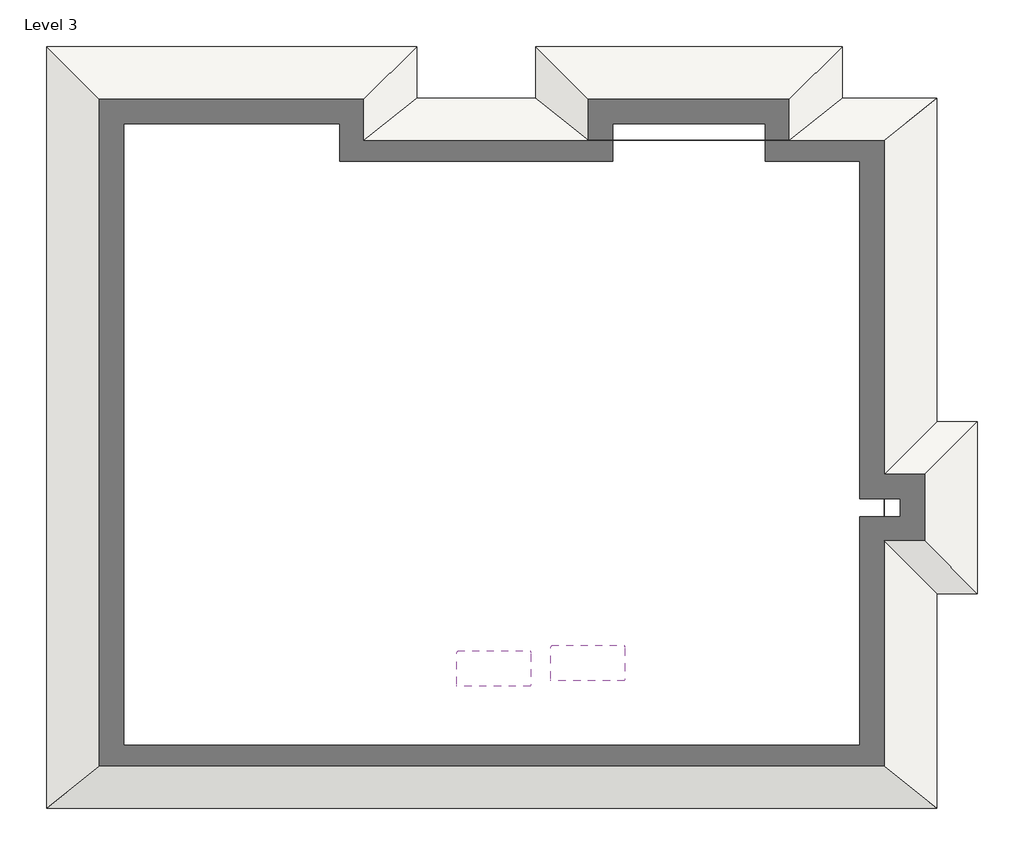
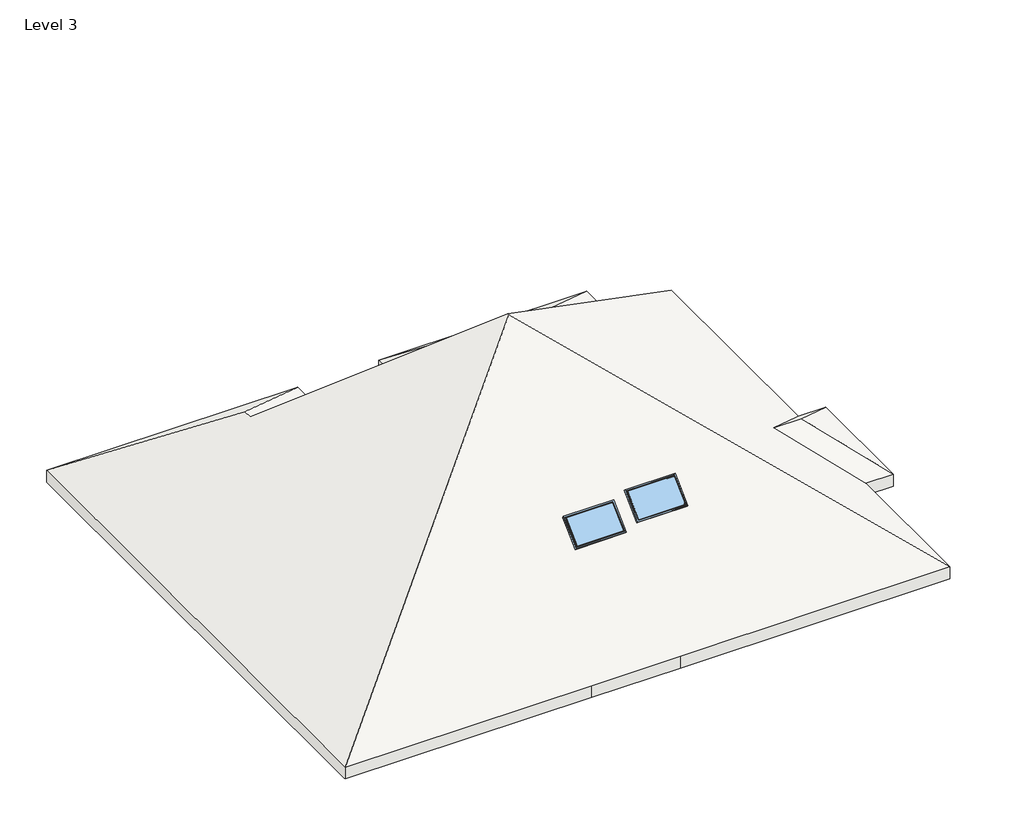
# One storey: 2 windows, 1 roof.
"""IFC4 building model written with IfcOpenShell, lengths in millimetres."""

from ifc_helpers import new_model, si_unit, origin, place, context, project, spatial, faceted_brep, transform, mapped, element, save
from components import m_skylight_top_hung_1500_x_900mm_68f14329

model = new_model("IFC4")

# Units and contexts
model_context = context("Model", 3, world=origin())
ifc_project = project(units=[si_unit("LENGTHUNIT", "METRE", prefix="MILLI")], contexts=[model_context])

# Site, building, storey
site = spatial("IfcSite", under=ifc_project)
building = spatial("IfcBuilding", under=site)
storey = spatial("IfcBuildingStorey", under=building, Name="Level 3", Elevation=6400.8)

# Roof
placement = place(None, origin())
element("IfcRoof", 1, ObjectType="Generic - 12\"", at=placement, inside=storey, context=model_context, shape_type="Brep", body=[
    faceted_brep([(-17511.6847893, 8702.9209401, 6400.8), (-25004.6847893, 8702.9209401, 6400.8), (-15823.7334075, 15996.7422903, 13286.5135363), (-15796.0361711, 15996.7422903, 13286.5135363), (-6615.0847893, 8702.9209401, 6400.8), (-14819.2847893, 8702.9209401, 6400.8), (-16452.8105951, 11516.8805107, 9057.3113917), (-15079.8105951, 11516.8805107, 9057.3113917), (-15079.8105951, 12078.9730536, 9587.9534304), (-16452.8105951, 12078.9730536, 9587.9534304), (-14509.5672436, 11633.6430926, 9167.5408109), (-13136.5672436, 11633.6430926, 9167.5408109), (-13136.5672436, 12195.7356355, 9698.1828496), (-14509.5672436, 12195.7356355, 9698.1828496), (-6615.0847893, 23290.5636405, 6400.8), (-6615.0847893, 16650.7922903, 6400.8), (-8393.0847893, 14872.7922903, 7734.3), (-6615.0847893, 13094.7922903, 6400.8), (-5776.8847893, 13094.7922903, 6400.8), (-7554.8847893, 14872.7922903, 7734.3), (-5776.8847893, 16650.7922903, 6400.8), (-8570.8847893, 24397.7922903, 6400.8), (-8570.8847893, 23330.9922903, 6400.8), (-8570.8847893, 23290.5636405, 6400.8), (-11736.8776369, 20775.3356139, 8775.2946357), (-11736.8776369, 21231.7994428, 8775.2946357), (-14902.8704844, 24397.7922903, 6400.8), (-17359.2847893, 24397.7922903, 6400.8), (-21181.9847893, 20575.0922903, 9267.825), (-25004.6847893, 24397.7922903, 6400.8), (-21181.9847893, 20253.6135777, 9267.825), (-17359.2847893, 23290.5636405, 6400.8), (-14902.8704844, 23290.5636405, 6400.8), (-14902.8704844, 23330.9922903, 6400.8), (-17359.2847893, 23330.9922903, 6400.8), (-17511.6847893, 8662.4922903, 6781.8), (-14819.2847893, 8662.4922903, 6781.8), (-6615.0847893, 8662.4922903, 6781.8), (-15809.8847893, 15967.3156971, 13677.9), (-25004.6847893, 8662.4922903, 6781.8), (-16452.8105951, 11307.6441674, 9278.948917), (-16452.8105951, 11869.7367103, 9809.5909557), (-15079.8105951, 11869.7367103, 9809.5909557), (-15079.8105951, 11307.6441674, 9278.948917), (-14509.5672436, 11424.4067493, 9389.1783362), (-14509.5672436, 11986.4992922, 9919.8203749), (-13136.5672436, 11986.4992922, 9919.8203749), (-13136.5672436, 11424.4067493, 9389.1783362), (-6615.0847893, 13094.7922903, 6781.8), (-8393.0847893, 14872.7922903, 8115.3), (-6615.0847893, 16650.7922903, 6781.8), (-6615.0847893, 23330.9922903, 6781.8), (-15809.8847893, 16026.1688835, 13677.9), (-5776.8847893, 13094.7922903, 6781.8), (-7554.8847893, 14872.7922903, 8115.3), (-5776.8847893, 16650.7922903, 6781.8), (-8570.8847893, 23330.9922903, 6781.8), (-8570.8847893, 24397.7922903, 6781.8), (-11736.8776369, 21231.7994428, 9156.2946357), (-11736.8776369, 20815.7642637, 9156.2946357), (-14902.8704844, 24397.7922903, 6781.8), (-17359.2847893, 24397.7922903, 6781.8), (-25004.6847893, 24397.7922903, 6781.8), (-21181.9847893, 20575.0922903, 9648.825), (-14902.8704844, 23330.9922903, 6781.8), (-17359.2847893, 23330.9922903, 6781.8), (-21181.9847893, 20294.0422275, 9648.825), (-14819.2847893, 8662.4922903, 6400.8), (-17511.6847893, 8662.4922903, 6400.8), (-6615.0847893, 8662.4922903, 6400.8), (-6615.0847893, 23330.9922903, 6400.8), (-25004.6847893, 8662.4922903, 6400.8)], [[[0, 1, 2, 3, 4, 5], [6, 7, 8, 9], [10, 11, 12, 13]], [[4, 3, 14, 15, 16, 17]], [[18, 17, 16, 19]], [[18, 19, 20]], [[21, 22, 23, 24, 25]], [[21, 25, 26]], [[27, 28, 29]], [[20, 19, 16, 15]], [[14, 3, 2, 30, 31, 32, 24, 23]], [[29, 28, 30, 2, 1]], [[32, 33, 26, 25, 24]], [[31, 30, 28, 27, 34]], [[35, 36, 37, 38, 39], [40, 41, 42, 43], [44, 45, 46, 47]], [[37, 48, 49, 50, 51, 52, 38]], [[48, 53, 54, 49]], [[53, 55, 54]], [[56, 57, 58, 59]], [[57, 60, 58]], [[61, 62, 63]], [[55, 50, 49, 54]], [[51, 56, 59, 64, 65, 66, 52]], [[62, 39, 38, 52, 66, 63]], [[60, 64, 59, 58]], [[65, 61, 63, 66]], [[67, 36, 35, 68]], [[69, 37, 36, 67]], [[17, 48, 37, 69, 4]], [[18, 53, 48, 17]], [[20, 55, 53, 18]], [[15, 50, 55, 20]], [[70, 51, 50, 15, 14]], [[22, 56, 51, 70]], [[21, 57, 56, 22]], [[26, 60, 57, 21]], [[33, 64, 60, 26]], [[34, 65, 64, 33]], [[27, 61, 65, 34]], [[29, 62, 61, 27]], [[71, 39, 62, 29, 1]], [[68, 35, 39, 71]], [[68, 71, 1, 0, 5, 4, 69, 67]], [[34, 33, 32, 31]], [[22, 70, 14, 23]], [[41, 40, 6, 9]], [[42, 41, 9, 8]], [[43, 42, 8, 7]], [[40, 43, 7, 6]], [[45, 44, 10, 13]], [[46, 45, 13, 12]], [[47, 46, 12, 11]], [[44, 47, 11, 10]]]),
])

# Windows
m_skylight_top_hung_1500_x_900mm_shape = m_skylight_top_hung_1500_x_900mm_68f14329(model_context)
element("IfcWindow", 2, ObjectType="M_Skylight-Top-Hung : 1500 x 900mm", at=placement, inside=storey, context=model_context, shape_type="MappedRepresentation", body=[
    mapped(m_skylight_top_hung_1500_x_900mm_shape, transform((-15766.3105951, 14308.7629022, 6662.9821073), x_axis=(-1.0, 0.0, 0.0), y_axis=(0.0, -0.7271572352921014, -0.6864709426933872), z_axis=(0.0, -0.6864709426933872, 0.7271572352921014))),
])
element("IfcWindow", 3, ObjectType="M_Skylight-Top-Hung : 1500 x 900mm", at=placement, inside=storey, context=model_context, shape_type="MappedRepresentation", body=[
    mapped(m_skylight_top_hung_1500_x_900mm_shape, transform((-13823.0672436, 14425.525484, 6773.2115264), x_axis=(-1.0, 0.0, 0.0), y_axis=(0.0, -0.7271572352921014, -0.6864709426933872), z_axis=(0.0, -0.6864709426933872, 0.7271572352921014))),
])

save(model, "model.ifc")

# Revit data of these elements
# Type "Generic - 12\""
#   Assembly Code = "B1020"
#   Layers, outside or top first: 1' - 0" no material (function 1)
# Type "M_Skylight-Top-Hung : 1500 x 900mm"
#   Type Mark = "23"
#   Fire Rating = "0.5h"
#   Assembly Code = "B2020100"
#   Analytic Construction = "Single-glazed windows - domestic"
#   Width = 4' - 11.05512"
#   Visual Light Transmittance = 0.9
#   Thermal Resistance (R) = 0.9899 (h·ft²·°F)/BTU
#   Solar Heat Gain Coefficient = 0.86
#   Rough Width = 4' - 11.64567"
#   Rough Height = 3' - 0.02362"
#   Height = 2' - 11.43307"
#   Heat Transfer Coefficient (U) = 1.0102 BTU/(h·ft²·°F)
#   Base Height = 0' - 3.14961"
#   Glass Panel Material = Glass
#   Frame Material = Metal - Bronze, Light Brush
# Element 1 (IfcRoof, "Generic - 12\"")
#   built-in parameter 1001705 = 44.875 (stored number, unit not read)
#   built-in parameter 1001710 = 33615
#   Phase Created = New Construction
#   Materials on its faces: "ROOF", "Default Roof"
# Element 2 (IfcWindow, "M_Skylight-Top-Hung : 1500 x 900mm")
#   Mark = "45"
#   Phase Created = New Construction
#   Materials on its faces: "Metal - Bronze, Light Brush", "Glass"
# Element 3 (IfcWindow, "M_Skylight-Top-Hung : 1500 x 900mm")
#   Mark = "46"
#   Phase Created = New Construction
#   Materials on its faces: "Metal - Bronze, Light Brush", "Glass"
# Materials
#   "Glass": class "Glass", colour RGB 0 128 192, transparency 0.75, Description = "Soda Lime Glass", Cost = 0
#   "Metal - Bronze, Light Brush": class "Metal", colour RGB 113 80 70, transparency 0
#   "ROOF": class "Generic", colour RGB 120 120 120, transparency 0, Cost = 0
#   "Default Roof": colour RGB 88 101 114, transparency 0, Cost = 0
